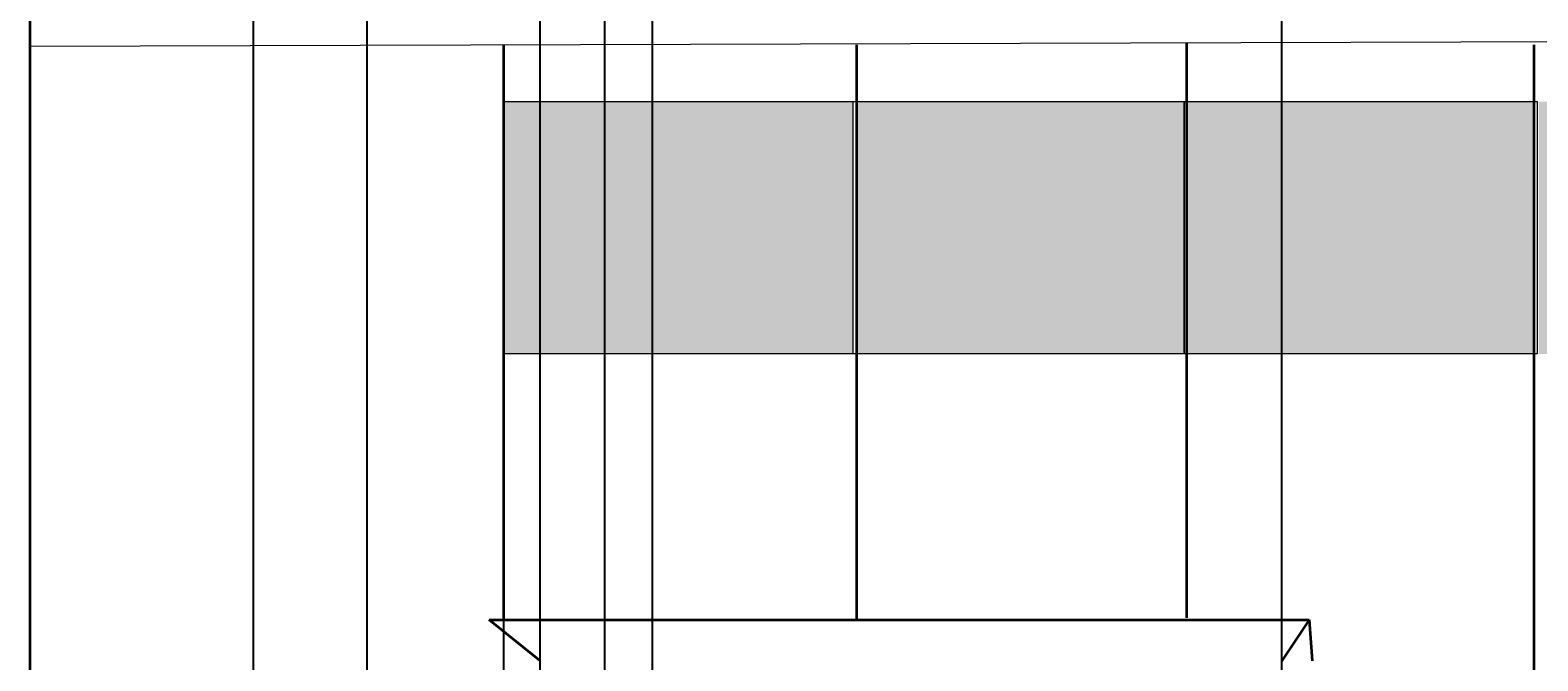
# Model space of a CAD drawing. Units: inches. Extents: x -26 to 776, y -22 to 650.
# Tile 35 of 62: x 192 to 309, y 504 to 554. Entities that reach past the tile are written whole.
import ezdxf

# ---------------------------------------------------------------- set-up
doc = ezdxf.new("R2010")
doc.units = ezdxf.units.IN
doc.header["$MEASUREMENT"] = 0
for name, color, linetype, lineweight in [('A-ANNO-DIMS', 2, 'Continuous', 18), ('A-GLAZ', 4, 'Continuous', 18), ('A-GLAZ-PATT', 9, 'Continuous', 13), ('A-ROOF', 7, 'Continuous', 35), ('A-WALL', 7, 'Continuous', 35), ('A-WALL-TRIM', 7, 'Continuous', 18)]:
    doc.layers.add(name, color=color, linetype=linetype, lineweight=lineweight)
doc.styles.get("Standard").update_dxf_attribs({"font": 'arial.ttf'})
doc.dimstyles.get("Standard").update_dxf_attribs({"dimtxt": 0.5625, "dimasz": 0.18, "dimexe": 0.18, "dimexo": 0.0625, "dimgap": 0.09, "dimtad": 0, "dimtih": 1, "dimtoh": 1, "dimdec": 4, "dimzin": 0, "dimdsep": 46, "dimlunit": 4, "dimtxsty": 'Standard', "dimcen": 0.09, "dimadec": 0, "dimazin": 0, "dimtfac": 1, "dimtdec": 4, "dimtofl": 0, "dimtmove": 0, "dimatfit": 3, "dimfxl": 1, "dimtolj": 1, "dimtzin": 0, "dimarcsym": 0})

# ---------------------------------------------------------------- blocks, each defined once
blk = doc.blocks.new('*D15')
at = {"layer": 'A-ANNO-DIMS', "color": 0, "lineweight": -2, "transparency": 16777216}
for p, q in [((11.11, 491.49), (11.11, 649.86)), ((231.42, 491.49), (231.42, 649.86)), ((11.29, 649.68), (120.22, 649.68)), ((231.24, 649.68), (122.31, 649.68))]:
    blk.add_line(p, q, dxfattribs=at)
at = {"layer": 'A-ANNO-DIMS', "color": 0, "transparency": 16777216}
for points in [[(11.29, 649.71), (11.29, 649.65), (11.11, 649.68)], [(231.24, 649.71), (231.24, 649.65), (231.42, 649.68)]]:
    blk.add_solid(points, dxfattribs=at)
at = {"layer": 'Defpoints', "color": 0, "transparency": 16777216}
for p in [(231.42, 649.68), (11.11, 491.43), (231.42, 491.43)]:
    blk.add_point(p, dxfattribs=at)
at = {"layer": 'A-ANNO-DIMS', "color": 0, "transparency": 16777216, "insert": (121.27, 649.68), "char_height": 0.562, "attachment_point": 5}
blk.add_mtext('\\A1;220.3', dxfattribs=at)
blk = doc.blocks.new('*D16')
at = {"layer": 'A-ANNO-DIMS', "color": 0, "lineweight": -2, "transparency": 16777216}
for p, q in [((231.42, 504.48), (231.42, 649.86)), ((289.24, 504.48), (289.24, 649.86)), ((231.6, 649.68), (259.3, 649.68)), ((289.06, 649.68), (261.37, 649.68))]:
    blk.add_line(p, q, dxfattribs=at)
at = {"layer": 'A-ANNO-DIMS', "color": 0, "transparency": 16777216}
for points in [[(231.6, 649.71), (231.6, 649.65), (231.42, 649.68)], [(289.06, 649.71), (289.06, 649.65), (289.24, 649.68)]]:
    blk.add_solid(points, dxfattribs=at)
at = {"layer": 'Defpoints', "color": 0, "transparency": 16777216}
for p in [(289.24, 649.68), (231.42, 504.42), (289.24, 504.42)]:
    blk.add_point(p, dxfattribs=at)
at = {"layer": 'A-ANNO-DIMS', "color": 0, "transparency": 16777216, "insert": (260.33, 649.68), "char_height": 0.562, "attachment_point": 5}
blk.add_mtext('\\A1;57.82', dxfattribs=at)
blk = doc.blocks.new('*D22')
at = {"layer": 'A-ANNO-DIMS', "color": 0, "lineweight": -2, "transparency": 16777216}
for p, q in [((22.89, 15.33), (22.89, 649.86)), ((217.95, 15.54), (217.95, 649.86)), ((23.07, 649.68), (119.19, 649.68)), ((217.77, 649.68), (121.65, 649.68))]:
    blk.add_line(p, q, dxfattribs=at)
at = {"layer": 'A-ANNO-DIMS', "color": 0, "transparency": 16777216}
for points in [[(23.07, 649.71), (23.07, 649.65), (22.89, 649.68)], [(217.77, 649.71), (217.77, 649.65), (217.95, 649.68)]]:
    blk.add_solid(points, dxfattribs=at)
at = {"layer": 'Defpoints', "color": 0, "transparency": 16777216}
for p in [(217.95, 649.68), (217.95, 15.48), (22.89, 15.27)]:
    blk.add_point(p, dxfattribs=at)
at = {"layer": 'A-ANNO-DIMS', "color": 0, "transparency": 16777216, "insert": (120.42, 649.68), "char_height": 0.562, "attachment_point": 5}
blk.add_mtext('\\A1;195.06', dxfattribs=at)
blk = doc.blocks.new('*D34')
at = {"layer": 'A-ANNO-DIMS', "color": 0, "lineweight": -2, "transparency": 16777216}
for p, q in [((228.57, 528.3), (228.57, -21.31)), ((357.3, 528.36), (357.3, -21.31)), ((228.75, -21.13), (291.71, -21.13)), ((357.12, -21.13), (294.17, -21.13))]:
    blk.add_line(p, q, dxfattribs=at)
at = {"layer": 'A-ANNO-DIMS', "color": 0, "transparency": 16777216}
for points in [[(228.75, -21.1), (228.75, -21.16), (228.57, -21.13)], [(357.12, -21.1), (357.12, -21.16), (357.3, -21.13)]]:
    blk.add_solid(points, dxfattribs=at)
at = {"layer": 'Defpoints', "color": 0, "transparency": 16777216}
for p in [(228.57, 528.36), (357.3, 528.42), (357.3, -21.13)]:
    blk.add_point(p, dxfattribs=at)
at = {"layer": 'A-ANNO-DIMS', "color": 0, "transparency": 16777216, "insert": (292.94, -21.13), "char_height": 0.562, "attachment_point": 5}
blk.add_mtext('\\A1;128.73', dxfattribs=at)
blk = doc.blocks.new('*D35')
at = {"layer": 'A-ANNO-DIMS', "color": 0, "lineweight": -2, "transparency": 16777216}
for p, q in [((82.13, 420.34), (82.13, 649.86)), ((209.09, 420.34), (209.09, 649.86)), ((82.31, 649.68), (144.38, 649.68)), ((208.91, 649.68), (146.84, 649.68))]:
    blk.add_line(p, q, dxfattribs=at)
at = {"layer": 'A-ANNO-DIMS', "color": 0, "transparency": 16777216}
for points in [[(82.31, 649.71), (82.31, 649.65), (82.13, 649.68)], [(208.91, 649.71), (208.91, 649.65), (209.09, 649.68)]]:
    blk.add_solid(points, dxfattribs=at)
at = {"layer": 'Defpoints', "color": 0, "transparency": 16777216}
for p in [(209.09, 649.68), (82.13, 420.28), (209.09, 420.28)]:
    blk.add_point(p, dxfattribs=at)
at = {"layer": 'A-ANNO-DIMS', "color": 0, "transparency": 16777216, "insert": (145.61, 649.68), "char_height": 0.562, "attachment_point": 5}
blk.add_mtext('\\A1;126.96', dxfattribs=at)
blk = doc.blocks.new('*D39')
at = {"layer": 'A-ANNO-DIMS', "color": 0, "lineweight": -2, "transparency": 16777216}
for p, q in [((289.24, 15.54), (289.24, 649.86)), ((425.74, 15.54), (425.74, 649.86)), ((289.42, 649.68), (356.48, 649.68)), ((425.56, 649.68), (358.51, 649.68))]:
    blk.add_line(p, q, dxfattribs=at)
at = {"layer": 'A-ANNO-DIMS', "color": 0, "transparency": 16777216}
for points in [[(289.42, 649.71), (289.42, 649.65), (289.24, 649.68)], [(425.56, 649.71), (425.56, 649.65), (425.74, 649.68)]]:
    blk.add_solid(points, dxfattribs=at)
at = {"layer": 'Defpoints', "color": 0, "transparency": 16777216}
for p in [(425.74, 649.68), (289.24, 15.48), (425.74, 15.48)]:
    blk.add_point(p, dxfattribs=at)
at = {"layer": 'A-ANNO-DIMS', "color": 0, "transparency": 16777216, "insert": (357.49, 649.68), "char_height": 0.562, "attachment_point": 5}
blk.add_mtext('\\A1;136.5', dxfattribs=at)
blk = doc.blocks.new('*D43')
at = {"layer": 'A-ANNO-DIMS', "color": 0, "lineweight": -2, "transparency": 16777216}
for p, q in [((231.42, 159.54), (231.42, 649.86)), ((236.46, 171.48), (236.46, 649.86)), ((231.6, 649.68), (233.13, 649.68)), ((236.28, 649.68), (234.76, 649.68))]:
    blk.add_line(p, q, dxfattribs=at)
at = {"layer": 'A-ANNO-DIMS', "color": 0, "transparency": 16777216}
for points in [[(231.6, 649.71), (231.6, 649.65), (231.42, 649.68)], [(236.28, 649.71), (236.28, 649.65), (236.46, 649.68)]]:
    blk.add_solid(points, dxfattribs=at)
at = {"layer": 'Defpoints', "color": 0, "transparency": 16777216}
for p in [(236.46, 649.68), (236.46, 171.42), (231.42, 159.48)]:
    blk.add_point(p, dxfattribs=at)
at = {"layer": 'A-ANNO-DIMS', "color": 0, "transparency": 16777216, "insert": (233.94, 649.68), "char_height": 0.562, "attachment_point": 5}
blk.add_mtext('\\A1;5.04', dxfattribs=at)
blk = doc.blocks.new('*D44')
at = {"layer": 'A-ANNO-DIMS', "color": 0, "lineweight": -2, "transparency": 16777216}
for p, q in [((231.42, 15.54), (231.42, 649.86)), ((240.17, 26.49), (240.17, 649.86)), ((231.6, 649.68), (234.98, 649.68)), ((239.99, 649.68), (236.61, 649.68))]:
    blk.add_line(p, q, dxfattribs=at)
at = {"layer": 'A-ANNO-DIMS', "color": 0, "transparency": 16777216}
for points in [[(231.6, 649.71), (231.6, 649.65), (231.42, 649.68)], [(239.99, 649.71), (239.99, 649.65), (240.17, 649.68)]]:
    blk.add_solid(points, dxfattribs=at)
at = {"layer": 'Defpoints', "color": 0, "transparency": 16777216}
for p in [(240.17, 649.68), (240.17, 26.42), (231.42, 15.48)]:
    blk.add_point(p, dxfattribs=at)
at = {"layer": 'A-ANNO-DIMS', "color": 0, "transparency": 16777216, "insert": (235.8, 649.68), "char_height": 0.562, "attachment_point": 5}
blk.add_mtext('\\A1;8.74', dxfattribs=at)

msp = doc.modelspace()

# ---------------------------------------------------------------- hatches: boundary and pattern name
at = {"layer": 'A-GLAZ-PATT'}
h = msp.add_hatch(dxfattribs=at)
h.set_pattern_fill('GOST_GLASS', color=256, scale=0.75)
h.set_pattern_definition([(45, (0, 0), (6.36396, 0), [3.75, -5.25]), (45, (1.591, 0), (6.36396, 0), [1.5, -7.5]), (45, (0, 1.591), (6.36396, 0), [1.5, -7.5])])
h.paths.add_polyline_path([(115.8402, 198.8773), (93.6448, 198.8773), (93.6448, 173.9734), (115.8402, 173.9734)])
h.paths.add_polyline_path([(144.1571, 198.8773), (115.8402, 198.8773), (115.8402, 173.9734), (144.1571, 173.9734)])
h.paths.add_polyline_path([(115.8402, 224.3396), (93.6448, 224.3396), (93.6448, 198.8773), (115.8402, 198.8773)])
h.paths.add_polyline_path([(144.1571, 248.4417), (115.8402, 248.4417), (115.8402, 224.3396), (144.1571, 224.3396)])
h.paths.add_polyline_path([(144.1571, 224.3396), (115.8402, 224.3396), (115.8402, 198.8773), (144.1571, 198.8773)])
h.paths.add_polyline_path([(170.5449, 224.3396), (144.1571, 224.3396), (144.1571, 198.8773), (170.5449, 198.8773)])
h.paths.add_polyline_path([(170.5449, 198.8773), (144.1571, 198.8773), (144.1571, 173.9734), (170.5449, 173.9734)])
h.paths.add_polyline_path([(194.6694, 198.8773), (170.5449, 198.8773), (170.5449, 173.9734), (194.6694, 173.9734)])
h.paths.add_polyline_path([(194.6694, 224.3396), (170.5449, 224.3396), (170.5449, 198.8773), (194.6694, 198.8773)])
h.paths.add_polyline_path([(194.6694, 248.4417), (170.5449, 248.4417), (170.5449, 224.3396), (194.6694, 224.3396)])
h.paths.add_polyline_path([(170.5449, 248.4417), (144.1571, 248.4417), (144.1571, 224.3396), (170.5449, 224.3396)])
h.paths.add_polyline_path([(144.1571, 269.3091), (115.8402, 269.3091), (115.8402, 248.4417), (144.1571, 248.4417)])
h.paths.add_polyline_path([(115.8402, 269.3091), (93.6448, 269.3091), (93.6448, 248.4417), (115.8402, 248.4417)])
h.paths.add_polyline_path([(115.8402, 248.4417), (93.6448, 248.4417), (93.6448, 224.3396), (115.8402, 224.3396)])
h.paths.add_polyline_path([(170.5449, 269.3091), (144.1571, 269.3091), (144.1571, 248.4417), (170.5449, 248.4417)])
h.paths.add_polyline_path([(194.6694, 269.3091), (170.5449, 269.3091), (170.5449, 248.4417), (194.6694, 248.4417)])
h.paths.add_polyline_path([(259.7413, 294.4171), (236.4647, 294.4171), (236.4647, 266.1888), (259.7413, 266.1888)])
h.paths.add_polyline_path([(285.0179, 294.4171), (261.7413, 294.4171), (261.7413, 266.1888), (285.0179, 266.1888)])
h.paths.add_polyline_path([(285.0179, 265.1888), (261.7413, 265.1888), (261.7413, 233.9172), (285.0179, 233.9172)])
h.paths.add_polyline_path([(259.7413, 265.1888), (236.4647, 265.1888), (236.4647, 233.9172), (259.7413, 233.9172)])
h.paths.add_polyline_path([(259.7413, 232.9172), (236.4647, 232.9172), (236.4647, 207.1741), (259.7413, 207.1741)])
h.paths.add_polyline_path([(285.0179, 232.9172), (261.7413, 232.9172), (261.7413, 207.1741), (285.0179, 207.1741)])
h.paths.add_polyline_path([(285.0179, 206.1741), (261.7413, 206.1741), (261.7413, 199.3298), (278.1134, 199.3298), (278.1134, 171.4173), (285.0179, 171.4173)])
h.paths.add_polyline_path([(259.7413, 206.1741), (236.4647, 206.1741), (236.4647, 199.3298), (259.7413, 199.3298)])
h.paths.add_polyline_path([(259.7413, 197.3298), (236.4647, 197.3298), (236.4647, 171.4173), (259.7413, 171.4173)])
h.paths.add_polyline_path([(276.1134, 197.3298), (261.7413, 197.3298), (261.7413, 171.4173), (276.1134, 171.4173)], flags=17)
h.paths.add_polyline_path([(255.8125, 548.0348), (228.5733, 548.0348), (228.5733, 528.3585), (255.8125, 528.3585)])
h.paths.add_polyline_path([(281.6181, 548.0348), (256.0792, 548.0348), (256.0792, 528.3585), (281.6181, 528.3585)])
h.paths.add_polyline_path([(308.8797, 548.0348), (281.789, 548.0348), (281.789, 528.3585), (308.8797, 528.3585)])
h.paths.add_polyline_path([(357.2724, 548.0995), (309.2457, 548.0348), (309.2457, 528.3585), (357.3034, 528.4233), (357.3034, 538.2614)])
h.paths.add_polyline_path([(259.7413, 437.1188), (236.4647, 437.1188), (236.4647, 408.8905), (259.7413, 408.8905)])
h.paths.add_polyline_path([(285.0179, 437.1188), (261.7413, 437.1188), (261.7413, 408.8905), (285.0179, 408.8905)])
h.paths.add_polyline_path([(259.7413, 407.8905), (236.4647, 407.8905), (236.4647, 376.6189), (259.7413, 376.6189)])
h.paths.add_polyline_path([(285.0179, 407.8905), (261.7413, 407.8905), (261.7413, 376.6189), (285.0179, 376.6189)])
h.paths.add_polyline_path([(285.0179, 375.6189), (261.7413, 375.6189), (261.7413, 349.8758), (285.0179, 349.8758)])
h.paths.add_polyline_path([(285.0179, 348.8758), (261.7413, 348.8758), (261.7413, 314.119), (285.0179, 314.119)])
h.paths.add_polyline_path([(259.7413, 348.8758), (236.4647, 348.8758), (236.4647, 314.119), (259.7413, 314.119)])
h.paths.add_polyline_path([(259.7413, 375.6189), (236.4647, 375.6189), (236.4647, 349.8758), (259.7413, 349.8758)])
h.paths.add_polyline_path([(194.6694, 404.1909), (170.5449, 404.1909), (170.5449, 383.3235), (194.6694, 383.3235)])
h.paths.add_polyline_path([(170.5449, 404.1909), (144.1571, 404.1909), (144.1571, 383.3235), (170.5449, 383.3235)])
h.paths.add_polyline_path([(144.1571, 404.1909), (115.8402, 404.1909), (115.8402, 383.3235), (144.1571, 383.3235)])
h.paths.add_polyline_path([(115.8402, 404.1909), (93.6448, 404.1909), (93.6448, 383.3235), (115.8402, 383.3235)])
h.paths.add_polyline_path([(115.8402, 383.3235), (93.6448, 383.3235), (93.6448, 359.2214), (115.8402, 359.2214)])
h.paths.add_polyline_path([(144.1571, 383.3235), (115.8402, 383.3235), (115.8402, 359.2214), (144.1571, 359.2214)])
h.paths.add_polyline_path([(115.8402, 359.2214), (93.6448, 359.2214), (93.6448, 333.7591), (115.8402, 333.7591)])
h.paths.add_polyline_path([(144.1571, 359.2214), (115.8402, 359.2214), (115.8402, 333.7591), (144.1571, 333.7591)])
h.paths.add_polyline_path([(115.8402, 333.7591), (93.6448, 333.7591), (93.6448, 308.8552), (115.8402, 308.8552)])
h.paths.add_polyline_path([(144.1571, 333.7591), (115.8402, 333.7591), (115.8402, 308.8552), (144.1571, 308.8552)])
h.paths.add_polyline_path([(170.5449, 333.7591), (144.1571, 333.7591), (144.1571, 308.8552), (170.5449, 308.8552)])
h.paths.add_polyline_path([(170.5449, 359.2214), (144.1571, 359.2214), (144.1571, 333.7591), (170.5449, 333.7591)])
h.paths.add_polyline_path([(170.5449, 383.3235), (144.1571, 383.3235), (144.1571, 359.2214), (170.5449, 359.2214)])
h.paths.add_polyline_path([(194.6694, 383.3235), (170.5449, 383.3235), (170.5449, 359.2214), (194.6694, 359.2214)])
h.paths.add_polyline_path([(194.6694, 359.2214), (170.5449, 359.2214), (170.5449, 333.7591), (194.6694, 333.7591)])
h.paths.add_polyline_path([(194.6694, 333.7591), (170.5449, 333.7591), (170.5449, 308.8552), (194.6694, 308.8552)])

# ---------------------------------------------------------------- linework, layer by layer
at = {"layer": 'A-GLAZ'}
for points in [[(228.5733, 548.0348), (256.0792, 548.0348), (256.0792, 528.3585), (228.5733, 528.3585)], [(255.8125, 548.0348), (281.6181, 548.0348), (281.6181, 528.3585), (255.8125, 528.3585)], [(281.6181, 548.0348), (309.124, 548.0348), (309.124, 528.3585), (281.6181, 528.3585)]]:
    msp.add_lwpolyline(points, close=True, dxfattribs=at)
at = {"layer": 'A-ROOF'}
for p, q in [((231.4249, 504.4205), (227.4501, 507.6108)), ((227.4501, 507.6108), (291.3688, 507.6108)), ((291.3688, 507.6108), (289.2424, 504.4205)), ((291.3688, 507.6108), (291.6017, 504.4205))]:
    msp.add_line(p, q, dxfattribs=at)
at = {"layer": 'A-WALL'}
for p, q in [((191.6782, 491.4269), (191.6782, 613.2713)), ((228.5733, 552.4655), (228.5733, 507.6108)), ((256.0792, 552.4655), (256.0792, 507.6108)), ((281.789, 552.6333), (281.789, 507.7786)), ((308.8797, 552.4655), (308.8797, 494.3612))]:
    msp.add_line(p, q, dxfattribs=at)
at = {"layer": 'A-WALL-TRIM'}
msp.add_line((191.6782, 552.3491), (357.2574, 552.8713), dxfattribs=at)

# ---------------------------------------------------------------- dimensions: what is measured, and where the dimension line sits
at = {"layer": 'A-ANNO-DIMS'}
for base, p1, p2, override, picture, middle in [((231.4249, 649.6763), (11.1074, 491.4269), (231.4249, 491.4269), {"dimdec": 1, "dimlfac": 1, "dimrnd": 0, "dimzin": 0, "dimdsep": 46, "dimlunit": 2}, '*D15', (121.2661, 649.6763)), ((217.9529, 649.6763), (22.8891, 15.2701), (217.9529, 15.4824), {"dimdec": 2, "dimlfac": 1, "dimrnd": 0, "dimzin": 0, "dimdsep": 46, "dimlunit": 2}, '*D22', (120.421, 649.6763)), ((209.091, 649.6763), (82.134, 420.2783), (209.091, 420.2783), {"dimdec": 2, "dimlfac": 1, "dimrnd": 0, "dimzin": 0, "dimdsep": 46, "dimlunit": 2}, '*D35', (145.6125, 649.6763)), ((289.2424, 649.6763), (231.4249, 504.4205), (289.2424, 504.4205), {"dimdec": 2, "dimlfac": 1, "dimrnd": 0, "dimzin": 0, "dimdsep": 46, "dimlunit": 2}, '*D16', (260.3336, 649.6763)), ((236.4647, 649.6763), (231.4249, 159.4824), (236.4647, 171.4173), {"dimdec": 2, "dimlfac": 1, "dimrnd": 0, "dimzin": 0, "dimdsep": 46, "dimlunit": 2}, '*D43', (233.9448, 649.6763)), ((240.1654, 649.6763), (231.4249, 15.4824), (240.1654, 26.4239), {"dimdec": 2, "dimlfac": 1, "dimrnd": 0, "dimzin": 0, "dimdsep": 46, "dimlunit": 2}, '*D44', (235.7952, 649.6763)), ((425.7434, 649.6763), (289.2424, 15.4824), (425.7434, 15.4824), {"dimdec": 1, "dimlfac": 1, "dimrnd": 0, "dimzin": 0, "dimdsep": 46, "dimlunit": 2}, '*D39', (357.4929, 649.6763)), ((357.3034, -21.1349), (228.5733, 528.3585), (357.3034, 528.4233), {"dimdec": 2, "dimlfac": 1, "dimrnd": 0, "dimzin": 0, "dimdsep": 46, "dimlunit": 2}, '*D34', (292.9384, -21.1349))]:
    dim = msp.add_linear_dim(base=base, p1=p1, p2=p2, dimstyle='Standard', override=override, dxfattribs=at)
    dim.commit()
    dim.dimension.update_dxf_attribs({"geometry": picture, "text_midpoint": middle})

doc.saveas('drawing.dxf')
